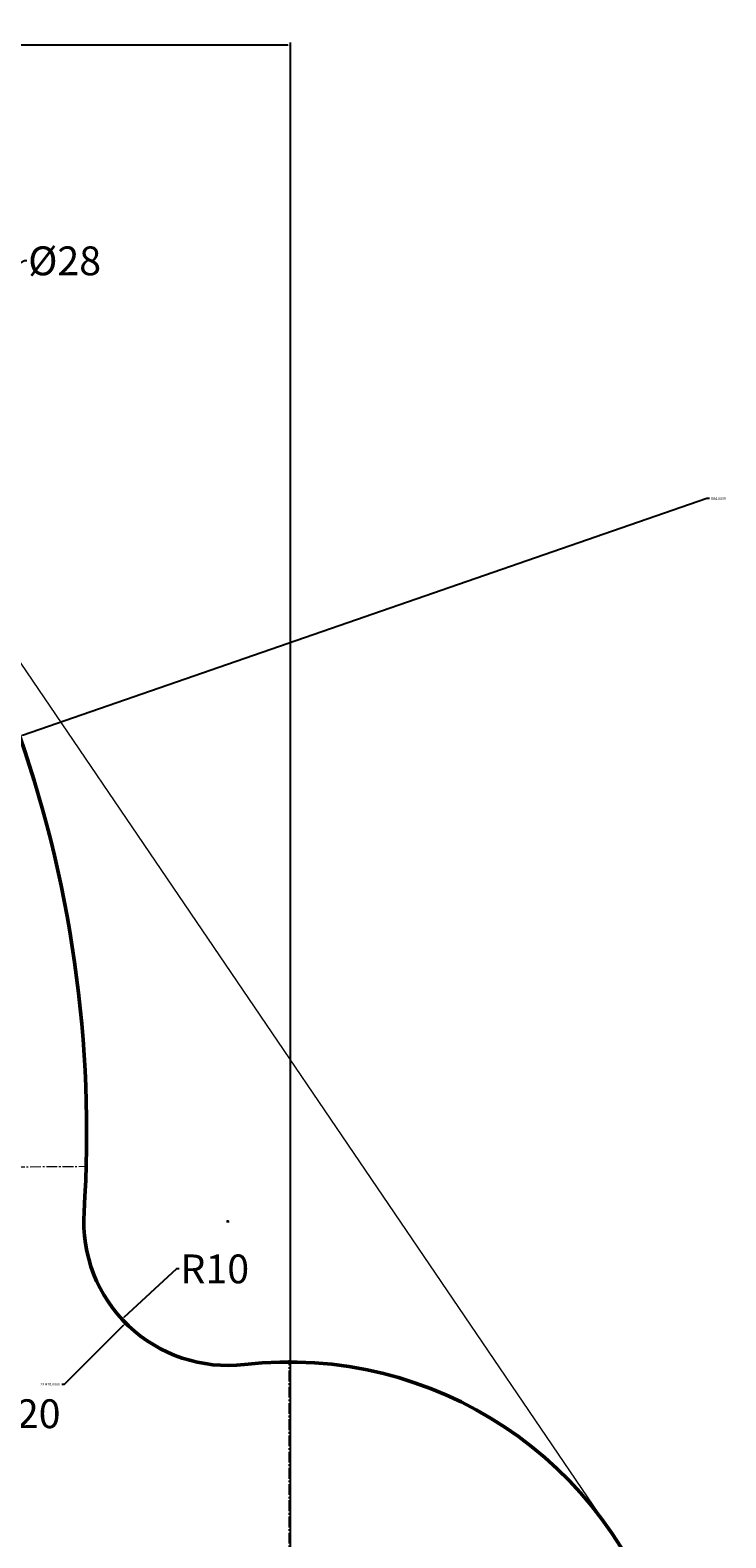
# Model space of a CAD drawing. Units: millimetres. Extents: x -60 to 113, y -37 to 126.
# Tile 17 of 17: x 49 to 98, y 21 to 126. Entities that reach past the tile are written whole.
import ezdxf

# ---------------------------------------------------------------- set-up
doc = ezdxf.new("R2010")
doc.units = ezdxf.units.MM
doc.header["$MEASUREMENT"] = 0
doc.linetypes.add('CENTER2', pattern=[1.125, 0.75, -0.125, 0.125, -0.125])
for name, color, linetype, lineweight in [('M-CNTR', 4, 'CENTER2', 18), ('M-CONS', 8, 'Continuous', 13), ('M-DIMS', 2, 'Continuous', 25), ('M-OUTL', 7, 'Continuous', 50)]:
    doc.layers.add(name, color=color, linetype=linetype, lineweight=lineweight)
doc.styles.get("Standard").update_dxf_attribs({"font": 'arial.ttf'})
doc.dimstyles.get("Standard").update_dxf_attribs({"dimtxt": 0.18, "dimasz": 0.18, "dimexe": 0.18, "dimexo": 0.0625, "dimgap": 0.09, "dimtad": 0, "dimtih": 1, "dimtoh": 1, "dimdec": 4, "dimzin": 0, "dimdsep": 46, "dimtxsty": 'Standard', "dimcen": 0.09, "dimadec": 0, "dimazin": 0, "dimtfac": 1, "dimtdec": 4, "dimtofl": 0, "dimtmove": 0, "dimatfit": 3, "dimfxl": 1, "dimtolj": 1, "dimtzin": 0, "dimarcsym": 0})

# ---------------------------------------------------------------- blocks, each defined once
blk = doc.blocks.new('*U3')
at = {"layer": 'M-CNTR', "color": 0, "transparency": 16777216}
blk.add_line((0, 5.4), (0, 27.12), dxfattribs=at)
blk = doc.blocks.new('*D8')
at = {"layer": 'Defpoints', "color": 0, "transparency": 16777216}
for p in [(23.98, 96.42), (-0.68, 83.15)]:
    blk.add_point(p, dxfattribs=at)
at = {"layer": 'M-DIMS', "color": 0, "lineweight": -2, "transparency": 16777216}
for p, q in [((48.91, 109.85), (24.14, 96.51)), ((49.09, 109.85), (48.91, 109.85)), ((11.56, 89.79), (11.74, 89.79)), ((11.65, 89.7), (11.65, 89.88))]:
    blk.add_line(p, q, dxfattribs=at)
at = {"layer": 'M-DIMS', "color": 0, "transparency": 16777216}
blk.add_solid([(24.12, 96.53), (24.15, 96.48), (23.98, 96.42)], dxfattribs=at)
at = {"layer": 'M-DIMS', "color": 0, "transparency": 16777216, "insert": (51.7, 109.85), "char_height": 0.18, "attachment_point": 5}
blk.add_mtext('\\A1;{\\H11.11111x;%%C28}', dxfattribs=at)
blk = doc.blocks.new('*D9')
at = {"layer": 'Defpoints', "color": 0, "transparency": 16777216}
for p in [(63.02, 43.2), (55.68, 36.41)]:
    blk.add_point(p, dxfattribs=at)
at = {"layer": 'M-DIMS', "color": 0, "lineweight": -2, "transparency": 16777216}
for p, q in [((59.46, 39.9), (55.81, 36.53)), ((59.64, 39.9), (59.46, 39.9))]:
    blk.add_line(p, q, dxfattribs=at)
at = {"layer": 'M-DIMS', "color": 0, "transparency": 16777216}
blk.add_solid([(55.79, 36.55), (55.83, 36.51), (55.68, 36.41)], dxfattribs=at)
at = {"layer": 'M-DIMS', "color": 0, "transparency": 16777216, "insert": (62.11, 39.9), "char_height": 0.18, "attachment_point": 5}
blk.add_mtext('\\A1;{\\H11.11111x;R10}', dxfattribs=at)
blk = doc.blocks.new('*D11')
at = {"layer": 'Defpoints', "color": 0, "transparency": 16777216}
for p in [(32.38, 55.74), (41.75, 38.07)]:
    blk.add_point(p, dxfattribs=at)
at = {"layer": 'M-DIMS', "color": 0, "lineweight": -2, "transparency": 16777216}
for p, q in [((36.97, 46.9), (37.15, 46.9)), ((37.06, 46.81), (37.06, 46.99)), ((46.11, 29.85), (41.83, 37.91)), ((46.29, 29.85), (46.11, 29.85))]:
    blk.add_line(p, q, dxfattribs=at)
at = {"layer": 'M-DIMS', "color": 0, "transparency": 16777216}
blk.add_solid([(41.86, 37.92), (41.81, 37.89), (41.75, 38.07)], dxfattribs=at)
at = {"layer": 'M-DIMS', "color": 0, "transparency": 16777216, "insert": (48.89, 29.85), "char_height": 0.18, "attachment_point": 5}
blk.add_mtext('\\A1;{\\H11.11111x;%%C20}', dxfattribs=at)
blk = doc.blocks.new('*D17')
at = {"layer": 'Defpoints', "color": 0, "transparency": 16777216}
for p in [(67.35, 124.82), (10.53, 88.53), (67.35, 6.44)]:
    blk.add_point(p, dxfattribs=at)
at = {"layer": 'M-DIMS', "color": 0, "lineweight": -2, "transparency": 16777216}
for p, q in [((10.53, 88.6), (10.53, 125)), ((10.71, 124.82), (37.42, 124.82)), ((67.17, 124.82), (40.47, 124.82)), ((67.35, 6.5), (67.35, 125))]:
    blk.add_line(p, q, dxfattribs=at)
at = {"layer": 'M-DIMS', "color": 0, "transparency": 16777216}
for points in [[(10.71, 124.85), (10.71, 124.79), (10.53, 124.82)], [(67.17, 124.85), (67.17, 124.79), (67.35, 124.82)]]:
    blk.add_solid(points, dxfattribs=at)
at = {"layer": 'M-DIMS', "color": 0, "transparency": 16777216, "insert": (38.94, 124.82), "char_height": 0.18, "attachment_point": 5}
blk.add_mtext('\\A1;{\\H11.11111x;56}', dxfattribs=at)
blk = doc.blocks.new('*D22')
at = {"layer": 'Defpoints', "color": 0, "transparency": 16777216}
for p in [(63.02, 43.2), (55.94, 36.14)]:
    blk.add_point(p, dxfattribs=at)
at = {"layer": 'M-DIMS', "color": 0, "lineweight": -2, "transparency": 16777216}
for p, q in [((62.93, 43.2), (63.11, 43.2)), ((63.02, 43.11), (63.02, 43.29)), ((51.69, 31.9), (55.81, 36.01)), ((51.51, 31.9), (51.69, 31.9))]:
    blk.add_line(p, q, dxfattribs=at)
at = {"layer": 'M-DIMS', "color": 0, "transparency": 16777216}
blk.add_solid([(55.79, 36.03), (55.83, 35.99), (55.94, 36.14)], dxfattribs=at)
at = {"layer": 'M-DIMS', "color": 0, "transparency": 16777216, "insert": (50.7, 31.9), "char_height": 0.18, "attachment_point": 5}
blk.add_mtext('\\A1;2X R10.0000', dxfattribs=at)
blk = doc.blocks.new('*D24')
at = {"layer": 'Defpoints', "color": 0, "transparency": 16777216}
for p in [(48.6, 76.85), (-30.78, 49.35)]:
    blk.add_point(p, dxfattribs=at)
at = {"layer": 'M-DIMS', "color": 0, "lineweight": -2, "transparency": 16777216}
for p, q in [((96.22, 93.35), (48.77, 76.91)), ((96.4, 93.35), (96.22, 93.35)), ((-30.87, 49.35), (-30.69, 49.35)), ((-30.78, 49.26), (-30.78, 49.44))]:
    blk.add_line(p, q, dxfattribs=at)
at = {"layer": 'M-DIMS', "color": 0, "transparency": 16777216}
blk.add_solid([(48.76, 76.94), (48.78, 76.88), (48.6, 76.85)], dxfattribs=at)
at = {"layer": 'M-DIMS', "color": 0, "transparency": 16777216, "insert": (97.02, 93.35), "char_height": 0.18, "attachment_point": 5}
blk.add_mtext('\\A1;R84.0000', dxfattribs=at)

msp = doc.modelspace()

# ---------------------------------------------------------------- linework, layer by layer
at = {"layer": 'M-CNTR'}
msp.add_line((18.93276, 46.7704), (53.1925, 47.02024), dxfattribs=at)
at = {"layer": 'M-CONS'}
msp.add_line((38.71594, 96.54155), (89.53778, 21.70335), dxfattribs=at)
at = {"layer": 'M-OUTL'}
for centre, radius, start, end in [((-30.77517, 49.3506), 84, 356.2470441, 43.4253235), ((63.02325, 43.19787), 10, 176.2470441, 276.5826838), ((67.26481, 6.44179), 27, 215.3846391, 96.5826838)]:
    msp.add_arc(centre, radius, start, end, dxfattribs=at)

# ---------------------------------------------------------------- block references
at = {"layer": 'M-CNTR'}
msp.add_blockref('*U3', (67.26481, 6.44179), dxfattribs=at)

# ---------------------------------------------------------------- dimensions: what is measured, and where the dimension line sits
at = {"layer": 'M-DIMS'}
dim = msp.add_linear_dim(base=(67.35481, 124.82251), p1=(10.53227, 88.53289), p2=(67.35481, 6.44179), text='{\\H11.11111x;56}', dimstyle='Standard', override={"dimclrd": 0, "dimclre": 0, "dimclrt": 0}, dxfattribs=at)
dim.commit()
dim.dimension.update_dxf_attribs({"geometry": '*D17', "text_midpoint": (38.94354, 124.82251)})
for p1, p2, text, picture, middle in [((-0.67791, 83.1508), (23.97668, 96.423), '{\\H11.11111x;%%C28}', '*D8', (51.70419, 109.84614)), ((32.37959, 55.73724), (41.74967, 38.06802), '{\\H11.11111x;%%C20}', '*D11', (48.8944, 29.85072))]:
    dim = msp.add_diameter_dim_2p(p1=p1, p2=p2, text=text, dimstyle='Standard', override={"dimclrd": 0, "dimclre": 0, "dimclrt": 0}, dxfattribs=at)
    dim.commit()
    dim.dimension.update_dxf_attribs({"geometry": picture, "text_midpoint": middle, "dimtype": 163})
dim = msp.add_radius_dim(center=(-30.77517, 49.3506), mpoint=(48.59582, 76.85052), dimstyle='Standard', override={"dimdec": 4, "dimlfac": 1, "dimrnd": 0, "dimzin": 0, "dimdsep": 46, "dimlunit": 2}, dxfattribs=at)
dim.commit()
dim.dimension.update_dxf_attribs({"geometry": '*D24', "text_midpoint": (97.01779, 93.35047), "dimtype": 164})
for mpoint, text, override, picture, middle in [((55.93957, 36.13943), '2X <>', {"dimdec": 4, "dimlfac": 1, "dimrnd": 0, "dimzin": 0, "dimdsep": 46, "dimlunit": 2}, '*D22', (50.69507, 31.90437)), ((55.682, 36.40772), '{\\H11.11111x;R10}', {"dimclrd": 0, "dimclre": 0, "dimclrt": 0}, '*D9', (62.11173, 39.89808))]:
    dim = msp.add_radius_dim(center=(63.02325, 43.19787), mpoint=mpoint, text=text, dimstyle='Standard', override=override, dxfattribs=at)
    dim.commit()
    dim.dimension.update_dxf_attribs({"geometry": picture, "text_midpoint": middle, "dimtype": 164})

doc.saveas('drawing.dxf')
